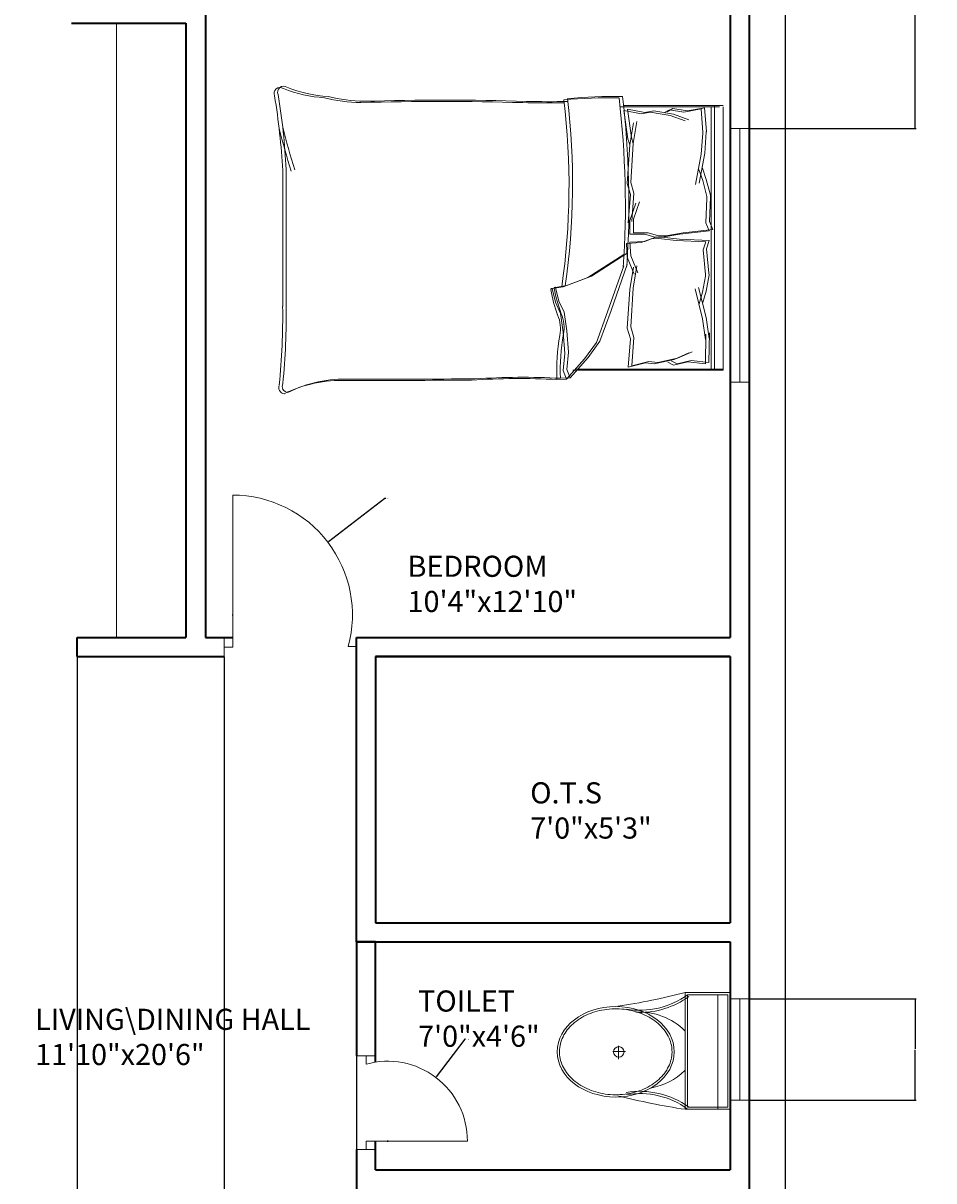
# Model space of a CAD drawing. Units: inches. Extents: x 1734 to 2405, y 1500 to 2491.
# Tile 12 of 14: x 1862 to 2078, y 2078 to 2352. Entities that reach past the tile are written whole.
import ezdxf

# ---------------------------------------------------------------- set-up
doc = ezdxf.new("R2010")
doc.units = ezdxf.units.IN
for name, color, linetype, lineweight in [('A-ANNO-DIMS', 2, 'Continuous', 18), ('A-AREA-IDEN', 7, 'Continuous', 18), ('A-DOOR', 3, 'Continuous', 18), ('A-FLOR-CASE', 9, 'Continuous', 18), ('A-FLOR-FIXT', 9, 'Continuous', 18), ('A-FURN', 8, 'Continuous', 13), ('A-GLAZ', 4, 'Continuous', 18), ('A-WALL', 7, 'Continuous', 35)]:
    doc.layers.add(name, color=color, linetype=linetype, lineweight=lineweight)
doc.styles.get("Standard").update_dxf_attribs({"font": 'arial.ttf'})
doc.dimstyles.get("Standard").update_dxf_attribs({"dimtxt": 0.18, "dimasz": 0.18, "dimexe": 0.18, "dimexo": 0.0625, "dimgap": 0.09, "dimtad": 0, "dimtih": 1, "dimtoh": 1, "dimdec": 4, "dimzin": 0, "dimdsep": 46, "dimtxsty": 'Standard', "dimcen": 0.09, "dimadec": 0, "dimazin": 0, "dimtfac": 1, "dimtdec": 4, "dimtofl": 0, "dimtmove": 0, "dimatfit": 3, "dimfxl": 1, "dimtolj": 1, "dimtzin": 0, "dimarcsym": 0})

# ---------------------------------------------------------------- blocks, each defined once
blk = doc.blocks.new('A$C31115884')
for p, q in [((257.5, 466.4), (257.5, 523.2)), ((283.1, 497.7), (223.4, 497.7)), ((0, 200), (0, 0)), ((520, 200), (0, 200)), ((10, 190), (10, 10)), ((510, 190), (10, 190)), ((510, 10), (510, 190)), ((520, 0), (520, 200)), ((510, 54.5), (0, 54.5)), ((10, 10), (510, 10)), ((0, 0), (520, 0))]:
    blk.add_line(p, q)
blk.add_circle((255.6, 496.4), 23.6)
for centre, radius, start, end in [((2777.7, -204.6), 2807, 165.4549, 171.7133), ((-294.5, 403.3), 374.7, 324.2091, 9.3499), ((3237, 905), 2807, 188.2867, 194.5451), ((-294.5, 403.3), 364.7, 324.2091, 9.3499), ((139.5, 406.2), 293.5, 315.8436, 2.6563), ((805.8, 403.3), 364.7, 170.6501, 215.7909), ((805.8, 403.3), 374.7, 179.2036, 215.7909), ((383.6, 406.2), 293.5, 190.2774, 224.1564)]:
    blk.add_arc(centre, radius, start, end)
blk.add_ellipse((256.2, 509.9), major_axis=(0, -260.7), ratio=0.772727)
blk.add_open_spline([(256.2, 259.2), (263.1, 259.2), (270, 259.7), (287.8, 262.3), (298.7, 265.1), (319.9, 273.1), (330.2, 278.4), (350.1, 291.1), (359.7, 298.7), (377.7, 315.9), (386.2, 325.5), (401.7, 346.6), (408.8, 358.1), (421.3, 382.5), (426.8, 395.5), (435.9, 422.4), (439.5, 436.4), (444.8, 465.1), (446.5, 479.7), (447.9, 509.2), (447.6, 524), (445, 553.3), (442.7, 567.8), (436.3, 596), (432.1, 609.7), (421.9, 636), (416, 648.6), (402.5, 672.1), (395, 683), (378.6, 703), (369.8, 712.1), (351.1, 728), (341.3, 734.8), (320.9, 746.2), (310.4, 750.7), (288.9, 757.3), (278, 759.4), (256, 761), (245, 760.6), (223.1, 757.2), (212.3, 754.3), (191.1, 746.1), (180.8, 740.7), (160.9, 727.8), (151.4, 720.1), (133.5, 702.7), (125.1, 693), (109.6, 671.7), (102.6, 660.2), (90.2, 635.7), (84.9, 622.7), (76, 595.6), (72.4, 581.6), (67.2, 552.9), (65.6, 538.2), (64.4, 508.8), (64.8, 494), (67.5, 464.7), (69.9, 450.2), (76.6, 422), (80.8, 408.3), (91.1, 382.2), (97.2, 369.7), (110.8, 346.3), (118.4, 335.4), (134.8, 315.6), (143.7, 306.7), (162.4, 290.9), (172.3, 284.2), (192.8, 273), (203.3, 268.6), (224.8, 262.2), (235.8, 260.2), (249.9, 259.3), (253, 259.2), (256.2, 259.2)], degree=3, knots=[0, 0, 0, 0, 0.110105, 0.110105, 0.285049, 0.285049, 0.459994, 0.459994, 0.634938, 0.634938, 0.809882, 0.809882, 0.984827, 0.984827, 1.159771, 1.159771, 1.334715, 1.334715, 1.50966, 1.50966, 1.684604, 1.684604, 1.859549, 1.859549, 2.034493, 2.034493, 2.209437, 2.209437, 2.384382, 2.384382, 2.559326, 2.559326, 2.73427, 2.73427, 2.909215, 2.909215, 3.084159, 3.084159, 3.259103, 3.259103, 3.434048, 3.434048, 3.608992, 3.608992, 3.783936, 3.783936, 3.958881, 3.958881, 4.133825, 4.133825, 4.30877, 4.30877, 4.483714, 4.483714, 4.658658, 4.658658, 4.833603, 4.833603, 5.008547, 5.008547, 5.183491, 5.183491, 5.358436, 5.358436, 5.53338, 5.53338, 5.708324, 5.708324, 5.883269, 5.883269, 6.058213, 6.058213, 6.233158, 6.233158, 6.283185, 6.283185, 6.283185, 6.283185])
blk = doc.blocks.new('BED-DOUBLE')
for p, q in [((81.88, 67.96), (105.53, 67.96)), ((81.88, 67.96), (105.53, 67.96)), ((82.71, 68.26), (106.37, 68.26)), ((82.71, 68.26), (106.37, 68.26)), ((83.83, 60.38), (82.88, 67.03)), ((82.88, 67.03), (87.04, 66.28)), ((83.83, 60.38), (82.88, 67.03)), ((82.88, 67.03), (87.04, 66.28)), ((84.66, 60.68), (83.72, 67.33)), ((83.72, 67.33), (87.87, 66.58)), ((84.66, 60.68), (83.72, 67.33)), ((83.72, 67.33), (87.87, 66.58)), ((87.04, 66.28), (89.12, 66.66)), ((87.04, 66.28), (89.12, 66.66)), ((87.87, 66.58), (89.95, 66.95)), ((87.87, 66.58), (89.95, 66.95)), ((89.12, 66.66), (93.84, 65.9)), ((89.12, 66.66), (93.84, 65.9)), ((89.95, 66.95), (94.67, 66.2)), ((89.95, 66.95), (94.67, 66.2)), ((93.65, 67.22), (92.33, 66.47)), ((93.65, 67.22), (92.33, 66.47)), ((94.48, 67.52), (93.16, 66.77)), ((94.48, 67.52), (93.16, 66.77)), ((97.05, 66.66), (93.65, 67.22)), ((97.05, 66.66), (93.65, 67.22)), ((93.84, 65.9), (97.42, 64.58)), ((93.84, 65.9), (97.42, 64.58)), ((97.88, 66.95), (94.48, 67.52)), ((97.88, 66.95), (94.48, 67.52)), ((94.67, 66.2), (98.26, 64.88)), ((94.67, 66.2), (98.26, 64.88)), ((101.2, 67.41), (97.05, 66.66)), ((101.2, 67.41), (97.05, 66.66)), ((102.04, 67.71), (97.88, 66.95)), ((102.04, 67.71), (97.88, 66.95)), ((101.17, 67.41), (101.6, 61.81)), ((101.17, 67.41), (101.6, 61.82)), ((102.01, 67.7), (102.44, 62.11)), ((102.01, 67.7), (102.44, 62.11)), ((103.53, 67.96), (103.53, 5.54)), ((103.53, 67.96), (103.53, 5.54)), ((104.36, 68.26), (104.36, 5.84)), ((104.36, 68.26), (104.36, 5.84)), ((106.37, 5.54), (106.37, 67.96)), ((85.12, 64.16), (84.25, 58.9)), ((85.12, 64.16), (84.25, 58.9)), ((85.96, 64.46), (85.09, 59.2)), ((85.96, 64.46), (85.09, 59.2)), ((84.25, 58.9), (83.83, 60.38)), ((84.25, 58.9), (83.83, 60.38)), ((85.09, 59.2), (84.66, 60.68)), ((85.09, 59.2), (84.66, 60.68)), ((101.58, 61.68), (101.2, 56.68)), ((101.58, 61.68), (101.2, 56.68)), ((101.6, 61.82), (101.58, 61.68)), ((101.6, 61.81), (101.58, 61.68)), ((102.41, 61.98), (102.04, 56.98)), ((102.41, 61.98), (102.04, 56.98)), ((102.44, 62.11), (102.41, 61.98)), ((102.44, 62.11), (102.41, 61.98)), ((84.25, 58.9), (83.69, 49.74)), ((84.25, 58.9), (83.69, 49.74)), ((85.09, 59.2), (84.52, 50.04)), ((85.09, 59.2), (84.52, 50.04)), ((101.2, 56.68), (99.88, 49.51)), ((101.2, 56.68), (99.88, 49.51)), ((102.04, 56.98), (100.71, 49.81)), ((102.04, 56.98), (100.71, 49.81)), ((2.04, 52.82), (2.04, 20.68)), ((2.04, 52.82), (2.04, 20.68)), ((2.87, 53.12), (2.87, 20.98)), ((2.87, 53.12), (2.87, 20.98)), ((100.64, 53.1), (101.58, 50.45)), ((100.64, 53.1), (101.58, 50.45)), ((101.47, 53.4), (102.41, 50.75)), ((101.47, 53.39), (102.41, 50.75)), ((83.69, 49.74), (84.42, 47.18)), ((83.69, 49.74), (84.42, 47.18)), ((84.52, 50.04), (85.25, 47.48)), ((84.52, 50.04), (85.25, 47.48)), ((101.58, 50.45), (102.52, 46.68)), ((101.58, 50.45), (102.52, 46.68)), ((102.41, 50.75), (103.36, 46.98)), ((102.41, 50.75), (103.36, 46.98)), ((84.42, 47.18), (83.89, 40.48)), ((84.42, 47.18), (83.89, 40.48)), ((85.25, 47.48), (84.72, 40.78)), ((85.25, 47.48), (84.72, 40.78)), ((102.52, 46.68), (102.52, 46.26)), ((102.52, 46.68), (102.52, 46.26)), ((103.36, 46.98), (103.36, 46.56)), ((103.36, 46.98), (103.36, 46.56)), ((84.29, 41.02), (85.72, 45.13)), ((84.29, 41.02), (85.72, 45.12)), ((85.13, 41.32), (86.55, 45.42)), ((85.13, 41.32), (86.55, 45.42)), ((102.52, 46.26), (102.33, 40.45)), ((102.52, 46.26), (102.33, 40.45)), ((103.36, 46.56), (103.17, 40.75)), ((103.36, 46.56), (103.17, 40.75)), ((85.13, 38.11), (85.13, 41.32)), ((85.13, 38.11), (85.13, 41.32)), ((84.29, 37.81), (84.29, 41.02)), ((84.29, 37.81), (84.29, 41.02)), ((103.09, 38.56), (96.1, 37.81)), ((103.09, 38.56), (96.1, 37.81)), ((103.92, 38.86), (96.94, 38.11)), ((103.92, 38.86), (96.94, 38.11)), ((102.33, 40.45), (103.09, 38.56)), ((102.33, 40.45), (103.09, 38.56)), ((103.17, 40.75), (103.92, 38.86)), ((103.17, 40.75), (103.92, 38.86)), ((86.97, 35.76), (83.47, 35.54)), ((86.97, 35.76), (83.47, 35.54)), ((87.79, 37.81), (84.29, 37.81)), ((87.79, 37.81), (84.29, 37.81)), ((87.8, 36.06), (84.3, 35.84)), ((87.8, 36.06), (84.3, 35.84)), ((84.3, 35.84), (84.51, 32.63)), ((84.3, 35.84), (84.51, 32.64)), ((88.63, 38.11), (85.13, 38.11)), ((88.63, 38.11), (85.13, 38.11)), ((89.37, 36.67), (86.97, 35.76)), ((89.37, 36.67), (86.97, 35.76)), ((90.25, 37.05), (87.79, 37.81)), ((90.25, 37.05), (87.79, 37.81)), ((90.2, 36.96), (87.8, 36.06)), ((90.2, 36.96), (87.8, 36.06)), ((91.08, 37.35), (88.63, 38.11)), ((91.08, 37.35), (88.63, 38.11)), ((91.06, 36.77), (89.37, 36.67)), ((91.06, 36.77), (89.37, 36.67)), ((91.9, 37.07), (90.2, 36.96)), ((91.9, 37.07), (90.2, 36.96)), ((91.95, 37.05), (90.25, 37.05)), ((91.95, 37.05), (90.25, 37.05)), ((95.26, 36.28), (91.06, 36.77)), ((95.26, 36.28), (91.06, 36.77)), ((92.78, 37.35), (91.08, 37.35)), ((92.78, 37.35), (91.08, 37.35)), ((96.09, 36.57), (91.9, 37.07)), ((96.09, 36.58), (91.9, 37.07)), ((96.1, 37.81), (91.95, 37.05)), ((96.1, 37.81), (91.95, 37.05)), ((96.94, 38.11), (92.78, 37.35)), ((96.94, 38.11), (92.78, 37.35)), ((102.28, 35.96), (95.26, 36.28)), ((102.28, 35.96), (95.26, 36.28)), ((103.11, 36.26), (96.09, 36.58)), ((103.11, 36.26), (96.09, 36.57)), ((101.64, 34.03), (102.28, 35.96)), ((101.64, 34.03), (102.28, 35.96)), ((102.48, 34.33), (103.11, 36.26)), ((102.48, 34.33), (103.11, 36.26)), ((82.83, 32.98), (74.35, 27.51)), ((82.83, 32.98), (74.35, 27.51)), ((83.66, 33.28), (75.18, 27.8)), ((83.66, 33.28), (75.18, 27.8)), ((83.47, 35.54), (83.67, 32.34)), ((83.47, 35.54), (83.67, 32.34)), ((102.19, 28.24), (101.64, 34.03)), ((102.19, 28.24), (101.64, 34.03)), ((103.03, 28.54), (102.48, 34.33)), ((103.03, 28.54), (102.48, 34.33)), ((79, 19.42), (82.83, 30.31)), ((79, 19.41), (82.83, 30.3)), ((79.83, 19.71), (83.66, 30.6)), ((79.83, 19.71), (83.66, 30.6)), ((83.67, 32.34), (85.35, 28.33)), ((83.67, 32.34), (85.35, 28.33)), ((84.51, 32.64), (86.18, 28.63)), ((84.51, 32.63), (86.18, 28.62)), ((85.96, 30.27), (85.09, 25)), ((85.96, 30.27), (85.09, 25)), ((74.35, 27.51), (68.49, 25.28)), ((74.35, 27.51), (68.49, 25.28)), ((75.18, 27.8), (69.32, 25.58)), ((75.18, 27.8), (69.32, 25.58)), ((85.12, 29.97), (84.25, 24.7)), ((85.12, 29.97), (84.25, 24.7)), ((101.51, 24), (102.22, 27.83)), ((101.51, 24), (102.22, 27.83)), ((102.22, 27.83), (102.19, 28.24)), ((102.22, 27.83), (102.19, 28.24)), ((102.35, 24.3), (103.05, 28.12)), ((102.35, 24.3), (103.05, 28.12)), ((103.05, 28.12), (103.03, 28.54)), ((103.05, 28.12), (103.03, 28.54)), ((68.49, 25.28), (65.86, 24.88)), ((68.49, 25.28), (65.86, 24.88)), ((65.86, 24.88), (66.67, 21.64)), ((65.86, 24.88), (66.67, 21.64)), ((69.32, 25.58), (66.69, 25.17)), ((69.32, 25.58), (66.69, 25.17)), ((66.69, 25.17), (67.5, 21.94)), ((66.69, 25.17), (67.5, 21.94)), ((84.25, 24.7), (83.69, 15.55)), ((84.25, 24.7), (83.69, 15.55)), ((85.09, 25), (84.52, 15.84)), ((85.09, 25), (84.52, 15.85)), ((101.52, 17.76), (99.76, 24.83)), ((101.52, 17.76), (99.76, 24.83)), ((102.36, 18.05), (100.59, 25.13)), ((102.36, 18.05), (100.59, 25.13)), ((67.5, 21.94), (68.72, 19.31)), ((67.5, 21.94), (68.72, 19.31)), ((100.73, 21.3), (101.51, 24)), ((100.73, 21.3), (101.51, 24)), ((101.57, 21.6), (102.35, 24.3)), ((101.57, 21.6), (102.35, 24.3)), ((66.67, 21.64), (67.88, 19.01)), ((66.67, 21.64), (67.88, 19.01)), ((68.72, 19.31), (69.32, 14.86)), ((68.72, 19.31), (69.32, 14.86)), ((76.37, 12.13), (79, 19.42)), ((76.37, 12.13), (79, 19.41)), ((77.21, 12.43), (79.83, 19.71)), ((77.21, 12.43), (79.83, 19.71)), ((67.88, 19.01), (68.49, 14.56)), ((67.88, 19.01), (68.49, 14.56)), ((102.21, 12.8), (101.52, 17.76)), ((102.21, 12.8), (101.52, 17.76)), ((103.05, 13.09), (102.36, 18.05)), ((103.05, 13.09), (102.36, 18.05)), ((68.49, 14.56), (68.89, 9.5)), ((68.49, 14.56), (68.89, 9.5)), ((69.32, 14.86), (69.73, 9.8)), ((69.32, 14.86), (69.73, 9.8)), ((83.69, 15.55), (84.42, 12.99)), ((83.69, 15.55), (84.42, 12.99)), ((84.52, 15.85), (85.25, 13.28)), ((84.52, 15.84), (85.25, 13.28)), ((102.19, 7.05), (102.32, 14.11)), ((102.19, 7.05), (102.32, 14.11)), ((102.32, 14.11), (102.21, 12.8)), ((102.32, 14.11), (102.21, 12.8)), ((103.03, 7.35), (103.15, 14.4)), ((103.03, 7.35), (103.15, 14.4)), ((103.15, 14.4), (103.05, 13.09)), ((103.15, 14.4), (103.05, 13.09)), ((73.54, 8.29), (76.37, 12.13)), ((73.54, 8.29), (76.37, 12.13)), ((74.38, 8.59), (77.21, 12.43)), ((74.38, 8.59), (77.21, 12.43)), ((84.42, 12.99), (83.89, 6.28)), ((84.42, 12.99), (83.89, 6.28)), ((85.25, 13.28), (84.72, 6.58)), ((85.25, 13.28), (84.72, 6.58)), ((68.89, 9.5), (68.49, 5.46)), ((68.89, 9.5), (68.49, 5.46)), ((69.3, 3.45), (73.54, 8.29)), ((69.3, 3.45), (73.54, 8.29)), ((69.73, 9.8), (69.32, 5.76)), ((69.73, 9.8), (69.32, 5.76)), ((70.13, 3.75), (74.38, 8.59)), ((70.13, 3.75), (74.38, 8.59)), ((90.92, 7.35), (95.58, 8.4)), ((90.92, 7.35), (95.58, 8.4)), ((94.75, 8.1), (98.25, 9.64)), ((94.75, 8.1), (98.25, 9.64)), ((95.58, 8.4), (99.08, 9.94)), ((95.58, 8.4), (99.08, 9.94)), ((69.32, 5.76), (70.13, 3.75)), ((69.32, 5.76), (70.13, 3.75)), ((105.53, 5.54), (70.78, 5.54)), ((105.53, 5.54), (70.78, 5.54)), ((106.37, 5.84), (71.61, 5.84)), ((106.37, 5.84), (71.61, 5.84)), ((83.89, 6.28), (87.99, 7.3)), ((83.89, 6.28), (87.99, 7.3)), ((84.72, 6.58), (88.82, 7.6)), ((84.72, 6.58), (88.82, 7.59)), ((87.99, 7.3), (90.08, 7.05)), ((87.99, 7.3), (90.08, 7.05)), ((88.82, 7.6), (90.92, 7.35)), ((88.82, 7.59), (90.92, 7.35)), ((90.08, 7.05), (94.75, 8.1)), ((90.08, 7.05), (94.75, 8.1)), ((94.64, 6.77), (93.28, 7.44)), ((94.64, 6.77), (93.28, 7.44)), ((95.48, 7.07), (94.11, 7.74)), ((95.48, 7.07), (94.11, 7.74)), ((98, 7.54), (94.64, 6.77)), ((98, 7.54), (94.64, 6.77)), ((98.83, 7.84), (95.48, 7.07)), ((98.83, 7.84), (95.48, 7.07)), ((102.19, 7.05), (98, 7.54)), ((102.19, 7.05), (98, 7.54)), ((103.03, 7.35), (98.83, 7.84)), ((103.03, 7.35), (98.83, 7.84)), ((106.37, 5.54), (105.53, 5.54)), ((67.02, 3.35), (69.3, 3.45, 5.06)), ((67.02, 3.35), (69.3, 3.45, 5.06)), ((67.85, 3.65), (70.13, 3.75, 5.06)), ((67.85, 3.65), (70.13, 3.75, 5.06)), ((68.49, 5.46), (69.3, 3.45)), ((68.49, 5.46), (69.3, 3.45))]:
    blk.add_line(p, q)
for centre, radius, start, end in [((1.42, 71.08), 1.42, 56.1736, 203.4781), ((1.42, 71.08), 1.42, 56.1736, 203.4781), ((2.25, 71.38), 1.42, 56.1736, 203.4781), ((2.25, 71.38), 1.42, 56.1736, 203.4781), ((13.75, 100.79), 30.77, 247.9751, 266.652), ((13.75, 100.79), 30.77, 247.9751, 266.652), ((14.58, 101.08), 30.77, 247.9751, 266.652), ((14.58, 101.08), 30.77, 247.9751, 266.652), ((-156.77, 44.51), 159.02, 2.9958, 9.4091), ((-156.77, 44.51), 159.02, 2.9958, 9.4091), ((-155.93, 44.81), 159.02, 2.9958, 9.4091), ((-155.93, 44.81), 159.02, 2.9958, 9.4091), ((21.27, 107.63), 38.7, 256.0648, 268.9113), ((21.27, 107.63), 38.7, 256.0648, 268.9113), ((22.11, 107.93), 38.7, 256.0648, 268.9113), ((22.11, 107.93), 38.7, 256.0648, 268.9113), ((39.43, -560.7), 629.91, 88.22771, 91.71854), ((39.43, -560.7), 629.91, 88.22771, 91.71854), ((40.26, -560.4), 629.91, 88.22771, 91.71854), ((40.26, -560.4), 629.91, 88.22771, 91.71854), ((64.82, 291.01), 222.17, 268.4762, 271.0082), ((64.82, 291.01), 222.17, 268.4762, 271.0082), ((65.65, 291.31), 222.17, 268.4762, 271.0082), ((65.65, 291.31), 222.17, 268.4762, 271.0082), ((-98.62, 49.31), 168.5, 351.7845, 6.9006), ((-98.62, 49.31), 168.5, 351.7845, 6.9006), ((79.29, -38.73), 108.8, 88.7218, 95.604), ((79.29, -38.73), 108.8, 88.7218, 95.604), ((-97.79, 49.61), 168.5, 351.7845, 6.9006), ((-97.79, 49.61), 168.5, 351.7845, 6.9006), ((80.12, -38.43), 108.8, 88.7218, 95.604), ((80.12, -38.43), 108.8, 88.7218, 95.604), ((-132.23, 44.6), 215.46, 356.0865, 6.7821), ((-132.23, 44.6), 215.46, 356.0865, 6.7821), ((-131.4, 44.9), 215.46, 356.0865, 6.7821), ((-131.4, 44.9), 215.46, 356.0865, 6.7821), ((137.34, 95.29), 139.04, 193.3832, 197.7053), ((137.34, 95.29), 139.04, 193.3832, 197.7053), ((136.5, 94.99), 139.04, 193.3832, 197.7053), ((136.5, 94.99), 139.04, 193.3832, 197.7053), ((65.78, 24.65), 0.241, 70.2464, 181.1377), ((65.78, 24.65), 0.241, 70.2464, 181.1377), ((66.61, 24.95), 0.241, 70.2464, 181.1377), ((66.61, 24.95), 0.241, 70.2464, 181.1377), ((104.43, 32.11), 38.73, 190.6617, 199.8806), ((104.43, 32.11), 38.73, 190.6617, 199.8806), ((103.6, 31.81), 38.73, 190.6617, 199.8806), ((103.6, 31.81), 38.73, 190.6617, 199.8806), ((-171.71, 18.75), 173.75, 354.4998, 0.6351), ((-171.71, 18.75), 173.75, 354.4998, 0.6351), ((-170.87, 19.05), 173.75, 354.4998, 0.6351), ((-170.87, 19.05), 173.75, 354.4998, 0.6351), ((59.73, 15.37), 8.13, 348.6608, 23.7384), ((59.73, 15.37), 8.13, 348.6608, 23.7384), ((60.57, 15.67), 8.13, 348.6608, 23.7384), ((60.57, 15.67), 8.13, 348.6608, 23.7384), ((114.23, 5.46), 47.26, 169.8763, 182.5657), ((114.23, 5.46), 47.26, 169.8763, 182.5657), ((115.06, 5.76), 47.26, 169.8763, 182.5657), ((115.06, 5.76), 47.26, 169.8763, 182.5657), ((15.85, -26.97), 30.12, 87.4714, 116.4681), ((15.85, -26.97), 30.12, 87.4714, 116.4681), ((16.69, -26.67), 30.12, 87.4714, 116.4681), ((16.69, -26.67), 30.12, 87.4714, 116.4681), ((16.96, 5961.08), 5957.95, 270.002168, 270.286887), ((16.96, 5961.08), 5957.95, 270.002168, 270.286887), ((17.79, 5961.38), 5957.95, 270.002168, 270.286887), ((17.79, 5961.38), 5957.95, 270.002168, 270.286887), ((58.1, -165.55), 169.13, 86.9791, 93.8365), ((58.1, -165.55), 169.13, 86.9791, 93.8365), ((58.94, -165.25), 169.13, 86.9791, 93.8365), ((58.94, -165.25), 169.13, 86.9791, 93.8365), ((2.53, 1.44), 1.44, 152.6588, 266.02), ((2.53, 1.44), 1.44, 152.6588, 266.02), ((3.36, 1.73), 1.44, 152.6588, 266.02), ((3.36, 1.74), 1.44, 152.6588, 266.02)]:
    blk.add_arc(centre, radius, start, end)
blk = doc.blocks.new('WIN-60')
for p, q in [((0, 60), (4.5, 60)), ((4.5, 60), (2.25, 60)), ((2.25, 60), (2.25, 0)), ((2.25, 0), (0, 0)), ((0, 0), (4.5, 0))]:
    blk.add_line(p, q)
blk = doc.blocks.new('*D29')
at = {"layer": 'A-ANNO-DIMS', "color": 0, "lineweight": -2, "transparency": 16777216}
for p, q in [((2033.96, 2121.3), (2073.42, 2121.3)), ((2073.24, 2121.12), (2073.24, 2109.48)), ((2073.24, 2097.48), (2073.24, 2109.12)), ((2033.96, 2097.3), (2073.42, 2097.3))]:
    blk.add_line(p, q, dxfattribs=at)
at = {"layer": 'A-ANNO-DIMS', "color": 0, "transparency": 16777216}
for points in [[(2073.21, 2121.12), (2073.27, 2121.12), (2073.24, 2121.3)], [(2073.21, 2097.48), (2073.27, 2097.48), (2073.24, 2097.3)]]:
    blk.add_solid(points, dxfattribs=at)
at = {"layer": 'Defpoints', "color": 0, "transparency": 16777216}
for p in [(2033.89, 2121.3), (2073.24, 2121.3), (2033.89, 2097.3)]:
    blk.add_point(p, dxfattribs=at)
at = {"layer": 'A-ANNO-DIMS', "color": 0, "transparency": 16777216, "insert": (2073.24, 2109.3), "char_height": 0.18, "attachment_point": 5}
blk.add_mtext('\\A1;24', dxfattribs=at)
blk = doc.blocks.new('*D30')
at = {"layer": 'A-ANNO-DIMS', "color": 0, "lineweight": -2, "transparency": 16777216}
for p, q in [((2033.96, 2425.82), (2073.42, 2425.82)), ((2073.24, 2425.64), (2073.24, 2376.77)), ((2073.24, 2327.53), (2073.24, 2376.41)), ((2033.96, 2327.35), (2073.42, 2327.35))]:
    blk.add_line(p, q, dxfattribs=at)
at = {"layer": 'A-ANNO-DIMS', "color": 0, "transparency": 16777216}
for points in [[(2073.21, 2425.64), (2073.27, 2425.64), (2073.24, 2425.82)], [(2073.21, 2327.53), (2073.27, 2327.53), (2073.24, 2327.35)]]:
    blk.add_solid(points, dxfattribs=at)
at = {"layer": 'Defpoints', "color": 0, "transparency": 16777216}
for p in [(2033.89, 2425.82), (2073.24, 2425.82), (2033.89, 2327.35)]:
    blk.add_point(p, dxfattribs=at)
at = {"layer": 'A-ANNO-DIMS', "color": 0, "transparency": 16777216, "insert": (2073.24, 2376.59), "char_height": 0.18, "attachment_point": 5}
blk.add_mtext('\\A1;98.47', dxfattribs=at)
blk = doc.blocks.new('*D33')
at = {"layer": 'A-ANNO-DIMS', "color": 0, "lineweight": -2, "transparency": 16777216}
for p, q in [((1824.83, 2202.26), (1824.83, 1615.47)), ((1874.68, 2202.26), (1874.68, 1615.47)), ((1825.01, 1615.65), (1849.36, 1615.65)), ((1874.5, 1615.65), (1850.15, 1615.65))]:
    blk.add_line(p, q, dxfattribs=at)
at = {"layer": 'A-ANNO-DIMS', "color": 0, "transparency": 16777216}
for points in [[(1825.01, 1615.68), (1825.01, 1615.62), (1824.83, 1615.65)], [(1874.5, 1615.68), (1874.5, 1615.62), (1874.68, 1615.65)]]:
    blk.add_solid(points, dxfattribs=at)
at = {"layer": 'Defpoints', "color": 0, "transparency": 16777216}
for p in [(1824.83, 2202.32), (1874.68, 2202.32), (1874.68, 1615.65)]:
    blk.add_point(p, dxfattribs=at)
at = {"layer": 'A-ANNO-DIMS', "color": 0, "transparency": 16777216, "insert": (1849.76, 1615.65), "char_height": 0.18, "attachment_point": 5}
blk.add_mtext('\\A1;49.84', dxfattribs=at)
blk = doc.blocks.new('*D34')
at = {"layer": 'A-ANNO-DIMS', "color": 0, "lineweight": -2, "transparency": 16777216}
for p, q in [((1940.89, 2204.68), (1940.89, 1615.47)), ((1909.52, 2202.26), (1909.52, 1615.47)), ((1909.7, 1615.65), (1924.81, 1615.65)), ((1940.71, 1615.65), (1925.6, 1615.65))]:
    blk.add_line(p, q, dxfattribs=at)
at = {"layer": 'A-ANNO-DIMS', "color": 0, "transparency": 16777216}
for points in [[(1909.7, 1615.68), (1909.7, 1615.62), (1909.52, 1615.65)], [(1940.71, 1615.68), (1940.71, 1615.62), (1940.89, 1615.65)]]:
    blk.add_solid(points, dxfattribs=at)
at = {"layer": 'Defpoints', "color": 0, "transparency": 16777216}
for p in [(1940.89, 2204.75), (1909.52, 2202.32), (1940.89, 1615.65)]:
    blk.add_point(p, dxfattribs=at)
at = {"layer": 'A-ANNO-DIMS', "color": 0, "transparency": 16777216, "insert": (1925.21, 1615.65), "char_height": 0.18, "attachment_point": 5}
blk.add_mtext('\\A1;31.37', dxfattribs=at)
blk = doc.blocks.new('*D36')
at = {"layer": 'A-ANNO-DIMS', "color": 0, "lineweight": -2, "transparency": 16777216}
for p, q in [((2081.68, 2425.82), (2042.21, 2425.82)), ((2042.39, 2425.64), (2042.39, 2065.96)), ((2042.39, 1705.92), (2042.39, 2065.6)), ((2081.68, 1705.74), (2042.21, 1705.74))]:
    blk.add_line(p, q, dxfattribs=at)
at = {"layer": 'A-ANNO-DIMS', "color": 0, "transparency": 16777216}
for points in [[(2042.36, 2425.64), (2042.42, 2425.64), (2042.39, 2425.82)], [(2042.36, 1705.92), (2042.42, 1705.92), (2042.39, 1705.74)]]:
    blk.add_solid(points, dxfattribs=at)
at = {"layer": 'Defpoints', "color": 0, "transparency": 16777216}
for p in [(2042.39, 2425.82), (2081.74, 2425.82), (2081.74, 1705.74)]:
    blk.add_point(p, dxfattribs=at)
at = {"layer": 'A-ANNO-DIMS', "color": 0, "transparency": 16777216, "insert": (2042.39, 2065.78), "char_height": 0.18, "attachment_point": 5}
blk.add_mtext('\\A1;720.1', dxfattribs=at)
blk = doc.blocks.new('*D47')
at = {"layer": 'A-ANNO-DIMS', "color": 0, "lineweight": -2, "transparency": 16777216}
for p, q in [((1966.51, 2111.72), (1959.77, 2102.83)), ((1966.69, 2111.72), (1966.51, 2111.72)), ((1948.16, 2087.63), (1948.34, 2087.63)), ((1948.25, 2087.54), (1948.25, 2087.72))]:
    blk.add_line(p, q, dxfattribs=at)
at = {"layer": 'A-ANNO-DIMS', "color": 0, "transparency": 16777216}
blk.add_solid([(1959.75, 2102.85), (1959.8, 2102.82), (1959.66, 2102.69)], dxfattribs=at)
at = {"layer": 'Defpoints', "color": 0, "transparency": 16777216}
for p in [(1959.66, 2102.69), (1948.25, 2087.63)]:
    blk.add_point(p, dxfattribs=at)
at = {"layer": 'A-ANNO-DIMS', "color": 0, "transparency": 16777216, "insert": (1967.24, 2111.72), "char_height": 0.18, "attachment_point": 5}
blk.add_mtext('\\A1;R18.896', dxfattribs=at)
blk = doc.blocks.new('*D48')
at = {"layer": 'A-ANNO-DIMS', "color": 0, "lineweight": -2, "transparency": 16777216}
for p, q in [((1947.59, 2239.76), (1934.21, 2229.54)), ((1947.77, 2239.76), (1947.59, 2239.76)), ((1911.43, 2212.2), (1911.61, 2212.2)), ((1911.52, 2212.11), (1911.52, 2212.29))]:
    blk.add_line(p, q, dxfattribs=at)
at = {"layer": 'A-ANNO-DIMS', "color": 0, "transparency": 16777216}
blk.add_solid([(1934.19, 2229.56), (1934.23, 2229.51), (1934.07, 2229.43)], dxfattribs=at)
at = {"layer": 'Defpoints', "color": 0, "transparency": 16777216}
for p in [(1934.07, 2229.43), (1911.52, 2212.2)]:
    blk.add_point(p, dxfattribs=at)
at = {"layer": 'A-ANNO-DIMS', "color": 0, "transparency": 16777216, "insert": (1948.25, 2239.76), "char_height": 0.18, "attachment_point": 5}
blk.add_mtext('\\A1;R28.37', dxfattribs=at)

msp = doc.modelspace()

# ---------------------------------------------------------------- linework, layer by layer
at = {"layer": 'A-DOOR'}
for p, q in [((1911.5222, 2204.5746), (1911.5222, 2240.5746)), ((1909.5222, 2206.8246), (1909.5222, 2202.3246)), ((1909.5222, 2202.3246), (1909.5222, 2204.5746)), ((1909.5222, 2204.5746), (1911.5222, 2204.5746)), ((1940.8942, 2204.7456), (1938.8942, 2204.7456)), ((1940.8942, 2107.8246), (1945.3942, 2107.8246)), ((1945.3942, 2107.8246), (1943.1442, 2107.8246)), ((1943.1442, 2107.8246), (1943.1442, 2105.8246)), ((1943.1442, 2085.6314), (1943.1442, 2087.6314)), ((1943.1442, 2087.6314), (1967.1442, 2087.6314)), ((1940.8942, 2085.6314), (1945.3942, 2085.6314)), ((1945.3942, 2085.6314), (1943.1442, 2085.6314))]:
    msp.add_line(p, q, dxfattribs=at)
for centre, radius, start, end in [((1911.5222, 2212.2045), 28.3701, 344.75705, 90), ((1948.2485, 2087.6314), 18.8956, 0, 105.67233)]:
    msp.add_arc(centre, radius, start, end, dxfattribs=at)
at = {"layer": 'A-FLOR-CASE'}
msp.add_line((1883.9911, 2206.8246), (1883.9911, 2352.3246), dxfattribs=at)
at = {"layer": 'A-GLAZ'}
for p, q in [((2031.6442, 2121.2994), (2029.3942, 2121.2994)), ((2029.3942, 2121.2994), (2033.8942, 2121.2994)), ((2031.6442, 2097.2994), (2031.6442, 2121.2994)), ((2029.3942, 2097.2994), (2033.8942, 2097.2994)), ((2033.8942, 2097.2994), (2031.6442, 2097.2994))]:
    msp.add_line(p, q, dxfattribs=at)
at = {"layer": 'A-WALL'}
for p, q in [((2033.8942, 2425.8246), (2033.8942, 1798.8246)), ((2029.3942, 2421.3246), (2029.3942, 2206.8246)), ((1905.0875, 2356.8246), (1905.0875, 2206.8246)), ((1873.2951, 2352.3246), (1900.3942, 2352.3246)), ((1900.3942, 2352.3246), (1900.3942, 2206.8246)), ((1874.676, 2202.3246), (1874.676, 2206.8246)), ((1874.676, 2206.8246), (1900.3942, 2206.8246)), ((1905.0875, 2206.8246), (1911.5222, 2206.8246)), ((1940.8942, 2134.8246), (1940.8942, 2206.8246)), ((1940.8942, 2206.8246), (1943.4302, 2206.8246)), ((1941.7632, 2206.8246), (2029.3942, 2206.8246)), ((1874.676, 2202.3246), (1909.5222, 2202.3246)), ((1945.3942, 2202.3246), (2029.3942, 2202.3246)), ((2029.3942, 2202.3246), (1945.3942, 2202.3246)), ((1945.3942, 2202.3246), (1945.3942, 2139.3246)), ((2029.3942, 2202.3246), (2029.3942, 2139.3246)), ((1945.3942, 2139.3246), (2029.3942, 2139.3246)), ((1945.3942, 2134.8246), (1940.8942, 2134.8246)), ((1940.8942, 2134.8246), (2029.3942, 2134.8246)), ((1940.8942, 2134.8246), (1940.8942, 2107.8246)), ((1945.3942, 2106.3102), (1945.3942, 2134.8246)), ((2029.3942, 2134.8246), (2029.3942, 2080.8246)), ((1945.3942, 2080.8246), (1945.3942, 2087.6314)), ((1940.8942, 2085.6314), (1940.8942, 2076.3246)), ((1945.3942, 2080.8246), (2029.3942, 2080.8246))]:
    msp.add_line(p, q, dxfattribs=at)

# ---------------------------------------------------------------- block references
at = {"layer": 'A-FLOR-FIXT', "xscale": 0.0531771398825126, "yscale": 0.0531771398825126, "zscale": 0.0531771398825126, "rotation": 89.99999999999999}
msp.add_blockref('A$C31115884', (2029.3942, 2095.1455), dxfattribs=at)
at = {"layer": 'A-FURN'}
msp.add_blockref('BED-DOUBLE', (1921.33, 2264.59), dxfattribs=at)
at = {"layer": 'A-GLAZ'}
msp.add_blockref('WIN-60', (2029.394, 2267.351), dxfattribs=at)

# ---------------------------------------------------------------- texts
at = {"layer": 'A-AREA-IDEN', "char_height": 5, "attachment_point": 1}
for s, width, insert in [('BEDROOM\\P10\'4"x12\'10"', 181.479508, (1952.9562, 2226.2245)), ('O.T.S\\P7\'0"x5\'3"', 102.061048, (1982.0121, 2172.5747)), ('TOILET\\P7\'0"x4\'6"', 90.590148, (1955.4529, 2123.2824)), ('LIVING\\\\DINING HALL\\P11\'10"x20\'6"', 245.467336, (1864.7081, 2118.9545))]:
    msp.add_mtext_dynamic_manual_height_columns(s, width=width, gutter_width=12.5, heights=[0], dxfattribs=dict(at, insert=insert))

# ---------------------------------------------------------------- dimensions: what is measured, and where the dimension line sits
at = {"layer": 'A-ANNO-DIMS'}
for base, p1, p2, override, picture, middle in [((2073.2442, 2425.8246), (2033.8942, 2327.351), (2033.8942, 2425.8246), {"dimdec": 2, "dimlfac": 1, "dimrnd": 0, "dimzin": 0, "dimdsep": 46, "dimlunit": 2}, '*D30', (2073.2442, 2376.5878)), ((2042.3945, 2425.8246), (2081.7445, 1705.7415), (2081.7445, 2425.8246), {"dimdec": 1, "dimlfac": 1, "dimrnd": 0, "dimzin": 0, "dimdsep": 46, "dimlunit": 2}, '*D36', (2042.3945, 2065.783)), ((2073.2442, 2121.2994), (2033.8942, 2097.2994), (2033.8942, 2121.2994), {"dimdec": 0, "dimlfac": 1, "dimrnd": 0, "dimzin": 0, "dimdsep": 46, "dimlunit": 2}, '*D29', (2073.2442, 2109.2994))]:
    dim = msp.add_linear_dim(base=base, p1=p1, p2=p2, angle=90, dimstyle='Standard', override=override, dxfattribs=at)
    dim.commit()
    dim.dimension.update_dxf_attribs({"geometry": picture, "text_midpoint": middle})
for center, mpoint, override, picture, middle in [((1911.5222, 2212.2045), (1934.0663, 2229.4272), {"dimdec": 2, "dimlfac": 1, "dimrnd": 0, "dimzin": 0, "dimdsep": 46, "dimlunit": 2}, '*D48', (1948.2526, 2239.7609)), ((1948.2485, 2087.6314), (1959.6629, 2102.6899), {"dimdec": 3, "dimlfac": 1, "dimrnd": 0, "dimzin": 0, "dimdsep": 46, "dimlunit": 2}, '*D47', (1967.2412, 2111.7249))]:
    dim = msp.add_radius_dim(center=center, mpoint=mpoint, dimstyle='Standard', override=override, dxfattribs=at)
    dim.commit()
    dim.dimension.update_dxf_attribs({"geometry": picture, "text_midpoint": middle, "dimtype": 164})
for base, p1, p2, picture, middle in [((1940.8942, 1615.6468), (1909.5222, 2202.3246), (1940.8942, 2204.7456), '*D34', (1925.2082, 1615.6468)), ((1874.676, 1615.6468), (1824.8343, 2202.3246), (1874.676, 2202.3246), '*D33', (1849.7551, 1615.6468))]:
    dim = msp.add_linear_dim(base=base, p1=p1, p2=p2, dimstyle='Standard', override={"dimdec": 2, "dimlfac": 1, "dimrnd": 0, "dimzin": 0, "dimdsep": 46, "dimlunit": 2}, dxfattribs=at)
    dim.commit()
    dim.dimension.update_dxf_attribs({"geometry": picture, "text_midpoint": middle})

doc.saveas('drawing.dxf')
